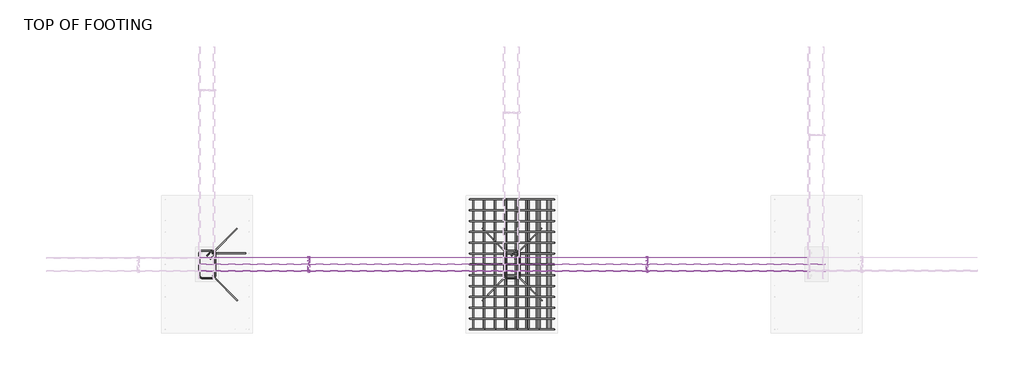
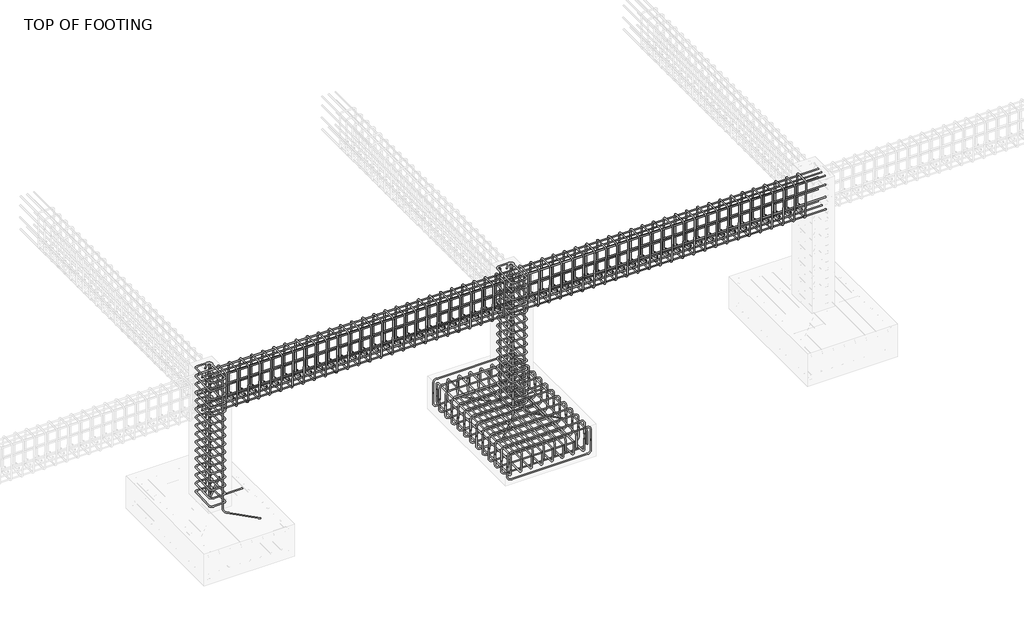
# One storey, part 3 of 21: 28 reinforcing bars.
"""IFC4 building model written with IfcOpenShell, lengths in millimetres."""

from ifc_helpers import new_model, si_unit, point, frame, origin, place, context, project, spatial, polyline, circle_curve, trimmed, segment, composite_curve, source, transform, mapped, element, save
from ifc_brep_helpers import swept_disk

model = new_model("IFC4")

# Units and contexts
model_context = context("Model", 3, world=origin())
ifc_project = project(units=[si_unit("LENGTHUNIT", "METRE", prefix="MILLI")], contexts=[model_context])

# Site, building, storey
site = spatial("IfcSite", under=ifc_project)
building = spatial("IfcBuilding", under=site)
storey = spatial("IfcBuildingStorey", under=building, Name="TOP OF FOOTING", Elevation=-1828.8)

# Reinforcing bars
placement = place(None, origin())
reinforcing_bar_shape = source(origin(), model_context, "Body", "SolidModel", [
    swept_disk(composite_curve([segment(polyline([(-5248.5313539, 443.1886958, -2045.4168622), (-5248.5313539, 443.1886958, -2192.7168622)]), True, "CONTINUOUS"), segment(trimmed(circle_curve(frame((-5294.8813539, 443.1886958, -2192.7168622), z_axis=(0.0, 1.0, 0.0), x_axis=(46.350000000000364, 0.0, 0.0)), 46.35), [point((-5248.5313539, 443.1886958, -2192.7168622))], [point((-5294.8813539, 443.1886958, -2239.0668622))], True, "CARTESIAN"), True, "CONTINUOUS"), segment(polyline([(-5294.8813539, 443.1886958, -2239.0668622), (-6309.4813539, 443.1886958, -2239.0668622)]), True, "CONTINUOUS"), segment(trimmed(circle_curve(frame((-6309.4813539, 443.1886958, -2192.7168622), z_axis=(0.0, 1.0, 0.0), x_axis=(0.0, 0.0, -46.34999999999991)), 46.35), [point((-6309.4813539, 443.1886958, -2239.0668622))], [point((-6355.8313539, 443.1886958, -2192.7168622))], True, "CARTESIAN"), True, "CONTINUOUS"), segment(polyline([(-6355.8313539, 443.1886958, -2192.7168622), (-6355.8313539, 443.1886958, -2045.4168622)]), True, "CONTINUOUS")], self_intersect=False), 6.35),
])
element("IfcReinforcingBar", 1, at=placement, inside=storey, context=model_context, shape_type="MappedRepresentation", body=[
    mapped(reinforcing_bar_shape, transform((0.0, 0.0, 0.0), x_axis=(1.0, 0.0, 0.0), y_axis=(0.0, 1.0, 0.0), z_axis=(0.0, 0.0, 1.0))),
    mapped(reinforcing_bar_shape, transform((0.0, -142.275, 0.0), x_axis=(1.0, 0.0, 0.0), y_axis=(0.0, 1.0, 0.0), z_axis=(0.0, 0.0, 1.0))),
    mapped(reinforcing_bar_shape, transform((0.0, -284.55, 0.0), x_axis=(1.0, 0.0, 0.0), y_axis=(0.0, 1.0, 0.0), z_axis=(0.0, 0.0, 1.0))),
    mapped(reinforcing_bar_shape, transform((0.0, -426.825, 0.0), x_axis=(1.0, 0.0, 0.0), y_axis=(0.0, 1.0, 0.0), z_axis=(0.0, 0.0, 1.0))),
    mapped(reinforcing_bar_shape, transform((0.0, -569.1, 0.0), x_axis=(1.0, 0.0, 0.0), y_axis=(0.0, 1.0, 0.0), z_axis=(0.0, 0.0, 1.0))),
    mapped(reinforcing_bar_shape, transform((0.0, -711.375, 0.0), x_axis=(1.0, 0.0, 0.0), y_axis=(0.0, 1.0, 0.0), z_axis=(0.0, 0.0, 1.0))),
    mapped(reinforcing_bar_shape, transform((0.0, -853.65, 0.0), x_axis=(1.0, 0.0, 0.0), y_axis=(0.0, 1.0, 0.0), z_axis=(0.0, 0.0, 1.0))),
    mapped(reinforcing_bar_shape, transform((0.0, -995.925, 0.0), x_axis=(1.0, 0.0, 0.0), y_axis=(0.0, 1.0, 0.0), z_axis=(0.0, 0.0, 1.0))),
    mapped(reinforcing_bar_shape, transform((0.0, -1138.2, 0.0), x_axis=(1.0, 0.0, 0.0), y_axis=(0.0, 1.0, 0.0), z_axis=(0.0, 0.0, 1.0))),
    mapped(reinforcing_bar_shape, transform((0.0, -1280.475, 0.0), x_axis=(1.0, 0.0, 0.0), y_axis=(0.0, 1.0, 0.0), z_axis=(0.0, 0.0, 1.0))),
    mapped(reinforcing_bar_shape, transform((0.0, -1422.75, 0.0), x_axis=(1.0, 0.0, 0.0), y_axis=(0.0, 1.0, 0.0), z_axis=(0.0, 0.0, 1.0))),
    mapped(reinforcing_bar_shape, transform((0.0, -1565.025, 0.0), x_axis=(1.0, 0.0, 0.0), y_axis=(0.0, 1.0, 0.0), z_axis=(0.0, 0.0, 1.0))),
    mapped(reinforcing_bar_shape, transform((0.0, -1707.3, 0.0), x_axis=(1.0, 0.0, 0.0), y_axis=(0.0, 1.0, 0.0), z_axis=(0.0, 0.0, 1.0))),
])
reinforcing_bar_2_shape = source(origin(), model_context, "Body", "SolidModel", [
    swept_disk(composite_curve([segment(polyline([(-6352.5002917, 443.1886958, -2057.1074344), (-6352.5002917, 443.1886958, -1909.8074344)]), True, "CONTINUOUS"), segment(trimmed(circle_curve(frame((-6306.1502917, 443.1886958, -1909.8074344), z_axis=(0.0, 1.0, 0.0), x_axis=(-46.350000000000364, 0.0, 0.0)), 46.35), [point((-6352.5002917, 443.1886958, -1909.8074344))], [point((-6306.1502917, 443.1886958, -1863.4574344))], True, "CARTESIAN"), True, "CONTINUOUS"), segment(polyline([(-6306.1502917, 443.1886958, -1863.4574344), (-5297.2599214, 443.1886958, -1863.4574344)]), True, "CONTINUOUS"), segment(trimmed(circle_curve(frame((-5297.2599214, 443.1886958, -1909.8074344), z_axis=(0.0, 1.0, 0.0), x_axis=(0.0, 0.0, 46.34999999999991)), 46.35), [point((-5297.2599214, 443.1886958, -1863.4574344))], [point((-5250.9099214, 443.1886958, -1909.8074344))], True, "CARTESIAN"), True, "CONTINUOUS"), segment(polyline([(-5250.9099214, 443.1886958, -1909.8074344), (-5250.9099214, 443.1886958, -2057.1074344)]), True, "CONTINUOUS")], self_intersect=False), 6.35),
])
element("IfcReinforcingBar", 2, at=placement, inside=storey, context=model_context, shape_type="MappedRepresentation", body=[
    mapped(reinforcing_bar_2_shape, transform((0.0, 0.0, 0.0), x_axis=(1.0, 0.0, 0.0), y_axis=(0.0, 1.0, 0.0), z_axis=(0.0, 0.0, 1.0))),
    mapped(reinforcing_bar_2_shape, transform((0.0, -142.275, 0.0), x_axis=(1.0, 0.0, 0.0), y_axis=(0.0, 1.0, 0.0), z_axis=(0.0, 0.0, 1.0))),
    mapped(reinforcing_bar_2_shape, transform((0.0, -284.55, 0.0), x_axis=(1.0, 0.0, 0.0), y_axis=(0.0, 1.0, 0.0), z_axis=(0.0, 0.0, 1.0))),
    mapped(reinforcing_bar_2_shape, transform((0.0, -426.825, 0.0), x_axis=(1.0, 0.0, 0.0), y_axis=(0.0, 1.0, 0.0), z_axis=(0.0, 0.0, 1.0))),
    mapped(reinforcing_bar_2_shape, transform((0.0, -569.1, 0.0), x_axis=(1.0, 0.0, 0.0), y_axis=(0.0, 1.0, 0.0), z_axis=(0.0, 0.0, 1.0))),
    mapped(reinforcing_bar_2_shape, transform((0.0, -711.375, 0.0), x_axis=(1.0, 0.0, 0.0), y_axis=(0.0, 1.0, 0.0), z_axis=(0.0, 0.0, 1.0))),
    mapped(reinforcing_bar_2_shape, transform((0.0, -853.65, 0.0), x_axis=(1.0, 0.0, 0.0), y_axis=(0.0, 1.0, 0.0), z_axis=(0.0, 0.0, 1.0))),
    mapped(reinforcing_bar_2_shape, transform((0.0, -995.925, 0.0), x_axis=(1.0, 0.0, 0.0), y_axis=(0.0, 1.0, 0.0), z_axis=(0.0, 0.0, 1.0))),
    mapped(reinforcing_bar_2_shape, transform((0.0, -1138.2, 0.0), x_axis=(1.0, 0.0, 0.0), y_axis=(0.0, 1.0, 0.0), z_axis=(0.0, 0.0, 1.0))),
    mapped(reinforcing_bar_2_shape, transform((0.0, -1280.475, 0.0), x_axis=(1.0, 0.0, 0.0), y_axis=(0.0, 1.0, 0.0), z_axis=(0.0, 0.0, 1.0))),
    mapped(reinforcing_bar_2_shape, transform((0.0, -1422.75, 0.0), x_axis=(1.0, 0.0, 0.0), y_axis=(0.0, 1.0, 0.0), z_axis=(0.0, 0.0, 1.0))),
    mapped(reinforcing_bar_2_shape, transform((0.0, -1565.025, 0.0), x_axis=(1.0, 0.0, 0.0), y_axis=(0.0, 1.0, 0.0), z_axis=(0.0, 0.0, 1.0))),
    mapped(reinforcing_bar_2_shape, transform((0.0, -1707.3, 0.0), x_axis=(1.0, 0.0, 0.0), y_axis=(0.0, 1.0, 0.0), z_axis=(0.0, 0.0, 1.0))),
])
reinforcing_bar_3_shape = source(origin(), model_context, "Body", "SolidModel", [
    swept_disk(composite_curve([segment(polyline([(-5294.4849216, 443.1886958, -2099.3509187), (-5294.4849216, 443.1886958, -1952.0509187)]), True, "CONTINUOUS"), segment(trimmed(circle_curve(frame((-5294.4849216, 396.8386958, -1952.0509187), z_axis=(1.0, 0.0, 0.0), x_axis=(0.0, 46.35000000000002, 0.0)), 46.35), [point((-5294.4849216, 443.1886958, -1952.0509187))], [point((-5294.4849216, 396.8386958, -1905.7009187))], True, "CARTESIAN"), True, "CONTINUOUS"), segment(polyline([(-5294.4849216, 396.8386958, -1905.7009187), (-5294.4849216, -1217.7613042, -1905.7009187)]), True, "CONTINUOUS"), segment(trimmed(circle_curve(frame((-5294.4849216, -1217.7613042, -1952.0509187), z_axis=(1.0, 0.0, 0.0), x_axis=(0.0, 0.0, 46.34999999999991)), 46.35), [point((-5294.4849216, -1217.7613042, -1905.7009187))], [point((-5294.4849216, -1264.1113042, -1952.0509187))], True, "CARTESIAN"), True, "CONTINUOUS"), segment(polyline([(-5294.4849216, -1264.1113042, -1952.0509187), (-5294.4849216, -1264.1113042, -2099.3509187)]), True, "CONTINUOUS")], self_intersect=False), 6.35),
])
element("IfcReinforcingBar", 3, at=placement, inside=storey, context=model_context, shape_type="MappedRepresentation", body=[
    mapped(reinforcing_bar_3_shape, transform((0.0, 0.0, 0.0), x_axis=(1.0, 0.0, 0.0), y_axis=(0.0, 1.0, 0.0), z_axis=(0.0, 0.0, 1.0))),
    mapped(reinforcing_bar_3_shape, transform((-145.0295561, 0.0, 0.0), x_axis=(1.0, 0.0, 0.0), y_axis=(0.0, 1.0, 0.0), z_axis=(0.0, 0.0, 1.0))),
    mapped(reinforcing_bar_3_shape, transform((-290.0591123, 0.0, 0.0), x_axis=(1.0, 0.0, 0.0), y_axis=(0.0, 1.0, 0.0), z_axis=(0.0, 0.0, 1.0))),
    mapped(reinforcing_bar_3_shape, transform((-435.0886684, 0.0, 0.0), x_axis=(1.0, 0.0, 0.0), y_axis=(0.0, 1.0, 0.0), z_axis=(0.0, 0.0, 1.0))),
    mapped(reinforcing_bar_3_shape, transform((-580.1182245, 0.0, 0.0), x_axis=(1.0, 0.0, 0.0), y_axis=(0.0, 1.0, 0.0), z_axis=(0.0, 0.0, 1.0))),
    mapped(reinforcing_bar_3_shape, transform((-725.1477807, 0.0, 0.0), x_axis=(1.0, 0.0, 0.0), y_axis=(0.0, 1.0, 0.0), z_axis=(0.0, 0.0, 1.0))),
    mapped(reinforcing_bar_3_shape, transform((-870.1773368, 0.0, 0.0), x_axis=(1.0, 0.0, 0.0), y_axis=(0.0, 1.0, 0.0), z_axis=(0.0, 0.0, 1.0))),
    mapped(reinforcing_bar_3_shape, transform((-1015.206893, 0.0, 0.0), x_axis=(1.0, 0.0, 0.0), y_axis=(0.0, 1.0, 0.0), z_axis=(0.0, 0.0, 1.0))),
])
reinforcing_bar_4_shape = source(origin(), model_context, "Body", "SolidModel", [
    swept_disk(composite_curve([segment(polyline([(-6309.6918146, 443.1886958, -2006.0306816), (-6309.6918146, 443.1886958, -2153.3306816)]), True, "CONTINUOUS"), segment(trimmed(circle_curve(frame((-6309.6918146, 396.8386958, -2153.3306816), z_axis=(-1.0, 0.0, 0.0), x_axis=(0.0, 46.35000000000002, 0.0)), 46.35), [point((-6309.6918146, 443.1886958, -2153.3306816))], [point((-6309.6918146, 396.8386958, -2199.6806816))], True, "CARTESIAN"), True, "CONTINUOUS"), segment(polyline([(-6309.6918146, 396.8386958, -2199.6806816), (-6309.6918146, -1217.7613042, -2199.6806816)]), True, "CONTINUOUS"), segment(trimmed(circle_curve(frame((-6309.6918146, -1217.7613042, -2153.3306816), z_axis=(-1.0, 0.0, 0.0), x_axis=(0.0, 0.0, -46.34999999999991)), 46.35), [point((-6309.6918146, -1217.7613042, -2199.6806816))], [point((-6309.6918146, -1264.1113042, -2153.3306816))], True, "CARTESIAN"), True, "CONTINUOUS"), segment(polyline([(-6309.6918146, -1264.1113042, -2153.3306816), (-6309.6918146, -1264.1113042, -2006.0306816)]), True, "CONTINUOUS")], self_intersect=False), 6.35),
])
element("IfcReinforcingBar", 4, at=placement, inside=storey, context=model_context, shape_type="MappedRepresentation", body=[
    mapped(reinforcing_bar_4_shape, transform((0.0, 0.0, 0.0), x_axis=(1.0, 0.0, 0.0), y_axis=(0.0, 1.0, 0.0), z_axis=(0.0, 0.0, 1.0))),
    mapped(reinforcing_bar_4_shape, transform((138.8823255, 0.0, 0.0), x_axis=(1.0, 0.0, 0.0), y_axis=(0.0, 1.0, 0.0), z_axis=(0.0, 0.0, 1.0))),
    mapped(reinforcing_bar_4_shape, transform((277.7646509, 0.0, 0.0), x_axis=(1.0, 0.0, 0.0), y_axis=(0.0, 1.0, 0.0), z_axis=(0.0, 0.0, 1.0))),
    mapped(reinforcing_bar_4_shape, transform((416.6469764, 0.0, 0.0), x_axis=(1.0, 0.0, 0.0), y_axis=(0.0, 1.0, 0.0), z_axis=(0.0, 0.0, 1.0))),
    mapped(reinforcing_bar_4_shape, transform((555.5293018, 0.0, 0.0), x_axis=(1.0, 0.0, 0.0), y_axis=(0.0, 1.0, 0.0), z_axis=(0.0, 0.0, 1.0))),
    mapped(reinforcing_bar_4_shape, transform((694.4116273, 0.0, 0.0), x_axis=(1.0, 0.0, 0.0), y_axis=(0.0, 1.0, 0.0), z_axis=(0.0, 0.0, 1.0))),
    mapped(reinforcing_bar_4_shape, transform((833.2939527, 0.0, 0.0), x_axis=(1.0, 0.0, 0.0), y_axis=(0.0, 1.0, 0.0), z_axis=(0.0, 0.0, 1.0))),
    mapped(reinforcing_bar_4_shape, transform((972.1762782, 0.0, 0.0), x_axis=(1.0, 0.0, 0.0), y_axis=(0.0, 1.0, 0.0), z_axis=(0.0, 0.0, 1.0))),
])
reinforcing_bar_5_shape = source(origin(), model_context, "Body", "SolidModel", [
    swept_disk(composite_curve([segment(polyline([(-9807.7927145, -296.7370695, -46.35), (-9752.0491515, -240.9935066, -46.35)]), True, "CONTINUOUS"), segment(trimmed(circle_curve(frame((-9729.8813539, -263.1613042, -46.35), z_axis=(0.0, 0.0, -1.0), x_axis=(-22.167797599999176, 22.16779760000003, 0.0)), 31.35), [point((-9752.0491515, -240.9935066, -46.35))], [point((-9698.5313539, -263.1613042, -46.35))], True, "CARTESIAN"), True, "CONTINUOUS"), segment(polyline([(-9698.5313539, -263.1613042, -46.35), (-9698.5313539, -557.7613042, -46.35)]), True, "CONTINUOUS"), segment(trimmed(circle_curve(frame((-9729.8813539, -557.7613042, -46.35), z_axis=(0.0, 0.0, -1.0), x_axis=(31.350000000000364, 0.0, 0.0)), 31.35), [point((-9698.5313539, -557.7613042, -46.35))], [point((-9729.8813539, -589.1113042, -46.35))], True, "CARTESIAN"), True, "CONTINUOUS"), segment(polyline([(-9729.8813539, -589.1113042, -46.35), (-9874.4813539, -589.1113042, -46.35)]), True, "CONTINUOUS"), segment(trimmed(circle_curve(frame((-9874.4813539, -557.7810893, -45.2363875), z_axis=(0.0, 0.035521928334481916, -0.9993688971583016), x_axis=(0.0, -31.330214899999987, -1.1136125000000021)), 31.35), [point((-9874.4813539, -589.1113042, -46.35))], [point((-9905.8313539, -557.7810893, -45.2363875))], True, "CARTESIAN"), True, "CONTINUOUS"), segment(polyline([(-9905.8313539, -557.7810893, -45.2363875), (-9905.8313539, -263.1415191, -34.7636125)]), True, "CONTINUOUS"), segment(trimmed(circle_curve(frame((-9874.4813539, -263.1415191, -34.7636125), z_axis=(0.0, 0.035521928334481916, -0.9993688971583016), x_axis=(-31.349999999998545, 0.0, 0.0)), 31.35), [point((-9905.8313539, -263.1415191, -34.7636125))], [point((-9874.4813539, -231.8113042, -33.65))], True, "CARTESIAN"), True, "CONTINUOUS"), segment(polyline([(-9874.4813539, -231.8113042, -33.65), (-9729.8813539, -231.8113042, -33.65)]), True, "CONTINUOUS"), segment(trimmed(circle_curve(frame((-9729.8813539, -263.1613042, -33.65), z_axis=(0.0, 0.0, -1.0), x_axis=(0.0, 31.350000000000023, 0.0)), 31.35), [point((-9729.8813539, -231.8113042, -33.65))], [point((-9707.7135563, -285.3291018, -33.65))], True, "CARTESIAN"), True, "CONTINUOUS"), segment(polyline([(-9707.7135563, -285.3291018, -33.65), (-9763.4571193, -341.0726647, -33.65)]), True, "CONTINUOUS")], self_intersect=False), 6.35),
])
element("IfcReinforcingBar", 5, at=placement, inside=storey, context=model_context, shape_type="MappedRepresentation", body=[
    mapped(reinforcing_bar_5_shape, transform((0.0, 0.0, 0.0), x_axis=(1.0, 0.0, 0.0), y_axis=(0.0, 1.0, 0.0), z_axis=(0.0, 0.0, 1.0))),
    mapped(reinforcing_bar_5_shape, transform((0.0, 0.0, -115.74), x_axis=(1.0, 0.0, 0.0), y_axis=(0.0, 1.0, 0.0), z_axis=(0.0, 0.0, 1.0))),
    mapped(reinforcing_bar_5_shape, transform((0.0, 0.0, -231.48), x_axis=(1.0, 0.0, 0.0), y_axis=(0.0, 1.0, 0.0), z_axis=(0.0, 0.0, 1.0))),
    mapped(reinforcing_bar_5_shape, transform((0.0, 0.0, -347.22), x_axis=(1.0, 0.0, 0.0), y_axis=(0.0, 1.0, 0.0), z_axis=(0.0, 0.0, 1.0))),
    mapped(reinforcing_bar_5_shape, transform((0.0, 0.0, -462.96), x_axis=(1.0, 0.0, 0.0), y_axis=(0.0, 1.0, 0.0), z_axis=(0.0, 0.0, 1.0))),
    mapped(reinforcing_bar_5_shape, transform((0.0, 0.0, -578.7), x_axis=(1.0, 0.0, 0.0), y_axis=(0.0, 1.0, 0.0), z_axis=(0.0, 0.0, 1.0))),
    mapped(reinforcing_bar_5_shape, transform((0.0, 0.0, -694.44), x_axis=(1.0, 0.0, 0.0), y_axis=(0.0, 1.0, 0.0), z_axis=(0.0, 0.0, 1.0))),
    mapped(reinforcing_bar_5_shape, transform((0.0, 0.0, -810.18), x_axis=(1.0, 0.0, 0.0), y_axis=(0.0, 1.0, 0.0), z_axis=(0.0, 0.0, 1.0))),
    mapped(reinforcing_bar_5_shape, transform((0.0, 0.0, -925.92), x_axis=(1.0, 0.0, 0.0), y_axis=(0.0, 1.0, 0.0), z_axis=(0.0, 0.0, 1.0))),
    mapped(reinforcing_bar_5_shape, transform((0.0, 0.0, -1041.66), x_axis=(1.0, 0.0, 0.0), y_axis=(0.0, 1.0, 0.0), z_axis=(0.0, 0.0, 1.0))),
    mapped(reinforcing_bar_5_shape, transform((0.0, 0.0, -1157.4), x_axis=(1.0, 0.0, 0.0), y_axis=(0.0, 1.0, 0.0), z_axis=(0.0, 0.0, 1.0))),
    mapped(reinforcing_bar_5_shape, transform((0.0, 0.0, -1273.14), x_axis=(1.0, 0.0, 0.0), y_axis=(0.0, 1.0, 0.0), z_axis=(0.0, 0.0, 1.0))),
    mapped(reinforcing_bar_5_shape, transform((0.0, 0.0, -1388.88), x_axis=(1.0, 0.0, 0.0), y_axis=(0.0, 1.0, 0.0), z_axis=(0.0, 0.0, 1.0))),
    mapped(reinforcing_bar_5_shape, transform((0.0, 0.0, -1504.62), x_axis=(1.0, 0.0, 0.0), y_axis=(0.0, 1.0, 0.0), z_axis=(0.0, 0.0, 1.0))),
    mapped(reinforcing_bar_5_shape, transform((0.0, 0.0, -1620.36), x_axis=(1.0, 0.0, 0.0), y_axis=(0.0, 1.0, 0.0), z_axis=(0.0, 0.0, 1.0))),
    mapped(reinforcing_bar_5_shape, transform((0.0, 0.0, -1736.1), x_axis=(1.0, 0.0, 0.0), y_axis=(0.0, 1.0, 0.0), z_axis=(0.0, 0.0, 1.0))),
])
element("IfcReinforcingBar", 6, at=placement, inside=storey, context=model_context, shape_type="SolidModel", body=[
    swept_disk(composite_curve([segment(polyline([(-9730.3607537, -262.059512, -40.0), (-9730.3607537, -262.059512, -1882.5259187)]), True, "CONTINUOUS"), segment(trimmed(circle_curve(frame((-9684.0107537, -262.059512, -1882.5259187), z_axis=(0.0, -1.0, 0.0), x_axis=(-46.350000000000364, 0.0, 0.0)), 46.35), [point((-9730.3607537, -262.059512, -1882.5259187))], [point((-9684.0107537, -262.059512, -1928.8759187))], True, "CARTESIAN"), True, "CONTINUOUS"), segment(polyline([(-9684.0107537, -262.059512, -1928.8759187), (-9294.4849216, -262.059512, -1928.8759187)]), True, "CONTINUOUS")], self_intersect=False), 6.35),
])
element("IfcReinforcingBar", 7, at=placement, inside=storey, context=model_context, shape_type="SolidModel", body=[
    swept_disk(composite_curve([segment(polyline([(-9730.3607537, -262.059512, -40.0), (-9730.3607537, -262.059512, -1882.5259187)]), True, "CONTINUOUS"), segment(trimmed(circle_curve(frame((-9697.9026361, -228.9718542, -1882.5259187), z_axis=(0.7138653253877265, -0.7002830122236834, 0.0), x_axis=(-32.45811760000106, -33.08765779999999, 0.0)), 46.35), [point((-9730.3607537, -262.059512, -1882.5259187))], [point((-9697.9026361, -228.9718542, -1928.8759187))], True, "CARTESIAN"), True, "CONTINUOUS"), segment(polyline([(-9697.9026361, -228.9718542, -1928.8759187), (-9413.1331156, 61.320903, -1928.8759187)]), True, "CONTINUOUS")], self_intersect=False), 6.35),
])
element("IfcReinforcingBar", 8, at=placement, inside=storey, context=model_context, shape_type="SolidModel", body=[
    swept_disk(composite_curve([segment(polyline([(-9725.3607537, -561.3630964, -40.0), (-9725.3607537, -561.3630964, -1882.5259187)]), True, "CONTINUOUS"), segment(trimmed(circle_curve(frame((-9692.9026361, -594.4507542, -1882.5259187), z_axis=(-0.7138653253877265, -0.7002830122236834, 0.0), x_axis=(-32.45811760000106, 33.08765779999999, 0.0)), 46.35), [point((-9725.3607537, -561.3630964, -1882.5259187))], [point((-9692.9026361, -594.4507542, -1928.8759187))], True, "CARTESIAN"), True, "CONTINUOUS"), segment(polyline([(-9692.9026361, -594.4507542, -1928.8759187), (-9408.1331156, -884.7435113, -1928.8759187)]), True, "CONTINUOUS")], self_intersect=False), 6.35),
])
reinforcing_bar_6_shape = source(origin(), model_context, "Body", "SolidModel", [
    swept_disk(composite_curve([segment(polyline([(-5807.7927145, -296.7370695, -46.35), (-5752.0491515, -240.9935066, -46.35)]), True, "CONTINUOUS"), segment(trimmed(circle_curve(frame((-5729.8813539, -263.1613042, -46.35), z_axis=(0.0, 0.0, -1.0), x_axis=(-22.167797600000085, 22.16779760000003, 0.0)), 31.35), [point((-5752.0491515, -240.9935066, -46.35))], [point((-5698.5313539, -263.1613042, -46.35))], True, "CARTESIAN"), True, "CONTINUOUS"), segment(polyline([(-5698.5313539, -263.1613042, -46.35), (-5698.5313539, -557.7613042, -46.35)]), True, "CONTINUOUS"), segment(trimmed(circle_curve(frame((-5729.8813539, -557.7613042, -46.35), z_axis=(0.0, 0.0, -1.0), x_axis=(31.350000000000364, 0.0, 0.0)), 31.35), [point((-5698.5313539, -557.7613042, -46.35))], [point((-5729.8813539, -589.1113042, -46.35))], True, "CARTESIAN"), True, "CONTINUOUS"), segment(polyline([(-5729.8813539, -589.1113042, -46.35), (-5874.4813539, -589.1113042, -46.35)]), True, "CONTINUOUS"), segment(trimmed(circle_curve(frame((-5874.4813539, -557.7810893, -45.2363875), z_axis=(0.0, 0.035521928334481916, -0.9993688971583016), x_axis=(0.0, -31.330214899999987, -1.1136125000000021)), 31.35), [point((-5874.4813539, -589.1113042, -46.35))], [point((-5905.8313539, -557.7810893, -45.2363875))], True, "CARTESIAN"), True, "CONTINUOUS"), segment(polyline([(-5905.8313539, -557.7810893, -45.2363875), (-5905.8313539, -263.1415191, -34.7636125)]), True, "CONTINUOUS"), segment(trimmed(circle_curve(frame((-5874.4813539, -263.1415191, -34.7636125), z_axis=(0.0, 0.035521928334481916, -0.9993688971583016), x_axis=(-31.350000000000364, 0.0, 0.0)), 31.35), [point((-5905.8313539, -263.1415191, -34.7636125))], [point((-5874.4813539, -231.8113042, -33.65))], True, "CARTESIAN"), True, "CONTINUOUS"), segment(polyline([(-5874.4813539, -231.8113042, -33.65), (-5729.8813539, -231.8113042, -33.65)]), True, "CONTINUOUS"), segment(trimmed(circle_curve(frame((-5729.8813539, -263.1613042, -33.65), z_axis=(0.0, 0.0, -1.0), x_axis=(0.0, 31.350000000000023, 0.0)), 31.35), [point((-5729.8813539, -231.8113042, -33.65))], [point((-5707.7135563, -285.3291018, -33.65))], True, "CARTESIAN"), True, "CONTINUOUS"), segment(polyline([(-5707.7135563, -285.3291018, -33.65), (-5763.4571193, -341.0726647, -33.65)]), True, "CONTINUOUS")], self_intersect=False), 6.35),
])
element("IfcReinforcingBar", 9, at=placement, inside=storey, context=model_context, shape_type="MappedRepresentation", body=[
    mapped(reinforcing_bar_6_shape, transform((0.0, 0.0, 0.0), x_axis=(1.0, 0.0, 0.0), y_axis=(0.0, 1.0, 0.0), z_axis=(0.0, 0.0, 1.0))),
    mapped(reinforcing_bar_6_shape, transform((0.0, 0.0, -115.74), x_axis=(1.0, 0.0, 0.0), y_axis=(0.0, 1.0, 0.0), z_axis=(0.0, 0.0, 1.0))),
    mapped(reinforcing_bar_6_shape, transform((0.0, 0.0, -231.48), x_axis=(1.0, 0.0, 0.0), y_axis=(0.0, 1.0, 0.0), z_axis=(0.0, 0.0, 1.0))),
    mapped(reinforcing_bar_6_shape, transform((0.0, 0.0, -347.22), x_axis=(1.0, 0.0, 0.0), y_axis=(0.0, 1.0, 0.0), z_axis=(0.0, 0.0, 1.0))),
    mapped(reinforcing_bar_6_shape, transform((0.0, 0.0, -462.96), x_axis=(1.0, 0.0, 0.0), y_axis=(0.0, 1.0, 0.0), z_axis=(0.0, 0.0, 1.0))),
    mapped(reinforcing_bar_6_shape, transform((0.0, 0.0, -578.7), x_axis=(1.0, 0.0, 0.0), y_axis=(0.0, 1.0, 0.0), z_axis=(0.0, 0.0, 1.0))),
    mapped(reinforcing_bar_6_shape, transform((0.0, 0.0, -694.44), x_axis=(1.0, 0.0, 0.0), y_axis=(0.0, 1.0, 0.0), z_axis=(0.0, 0.0, 1.0))),
    mapped(reinforcing_bar_6_shape, transform((0.0, 0.0, -810.18), x_axis=(1.0, 0.0, 0.0), y_axis=(0.0, 1.0, 0.0), z_axis=(0.0, 0.0, 1.0))),
    mapped(reinforcing_bar_6_shape, transform((0.0, 0.0, -925.92), x_axis=(1.0, 0.0, 0.0), y_axis=(0.0, 1.0, 0.0), z_axis=(0.0, 0.0, 1.0))),
    mapped(reinforcing_bar_6_shape, transform((0.0, 0.0, -1041.66), x_axis=(1.0, 0.0, 0.0), y_axis=(0.0, 1.0, 0.0), z_axis=(0.0, 0.0, 1.0))),
    mapped(reinforcing_bar_6_shape, transform((0.0, 0.0, -1157.4), x_axis=(1.0, 0.0, 0.0), y_axis=(0.0, 1.0, 0.0), z_axis=(0.0, 0.0, 1.0))),
    mapped(reinforcing_bar_6_shape, transform((0.0, 0.0, -1273.14), x_axis=(1.0, 0.0, 0.0), y_axis=(0.0, 1.0, 0.0), z_axis=(0.0, 0.0, 1.0))),
    mapped(reinforcing_bar_6_shape, transform((0.0, 0.0, -1388.88), x_axis=(1.0, 0.0, 0.0), y_axis=(0.0, 1.0, 0.0), z_axis=(0.0, 0.0, 1.0))),
    mapped(reinforcing_bar_6_shape, transform((0.0, 0.0, -1504.62), x_axis=(1.0, 0.0, 0.0), y_axis=(0.0, 1.0, 0.0), z_axis=(0.0, 0.0, 1.0))),
    mapped(reinforcing_bar_6_shape, transform((0.0, 0.0, -1620.36), x_axis=(1.0, 0.0, 0.0), y_axis=(0.0, 1.0, 0.0), z_axis=(0.0, 0.0, 1.0))),
    mapped(reinforcing_bar_6_shape, transform((0.0, 0.0, -1736.1), x_axis=(1.0, 0.0, 0.0), y_axis=(0.0, 1.0, 0.0), z_axis=(0.0, 0.0, 1.0))),
])
element("IfcReinforcingBar", 10, at=placement, inside=storey, context=model_context, shape_type="SolidModel", body=[
    swept_disk(composite_curve([segment(polyline([(-5730.3607537, -262.059512, -40.0), (-5730.3607537, -262.059512, -1882.5259187)]), True, "CONTINUOUS"), segment(trimmed(circle_curve(frame((-5684.0107537, -262.059512, -1882.5259187), z_axis=(0.0, -1.0, 0.0), x_axis=(-46.349999999999454, 0.0, 0.0)), 46.35), [point((-5730.3607537, -262.059512, -1882.5259187))], [point((-5684.0107537, -262.059512, -1928.8759187))], True, "CARTESIAN"), True, "CONTINUOUS"), segment(polyline([(-5684.0107537, -262.059512, -1928.8759187), (-5294.4849216, -262.059512, -1928.8759187)]), True, "CONTINUOUS")], self_intersect=False), 6.35),
])
element("IfcReinforcingBar", 11, at=placement, inside=storey, context=model_context, shape_type="SolidModel", body=[
    swept_disk(composite_curve([segment(polyline([(-5730.3607537, -262.059512, -40.0), (-5730.3607537, -262.059512, -1882.5259187)]), True, "CONTINUOUS"), segment(trimmed(circle_curve(frame((-5697.9026361, -228.9718542, -1882.5259187), z_axis=(0.7138653253877265, -0.7002830122236834, 0.0), x_axis=(-32.45811760000015, -33.08765779999999, 0.0)), 46.35), [point((-5730.3607537, -262.059512, -1882.5259187))], [point((-5697.9026361, -228.9718542, -1928.8759187))], True, "CARTESIAN"), True, "CONTINUOUS"), segment(polyline([(-5697.9026361, -228.9718542, -1928.8759187), (-5413.1331156, 61.320903, -1928.8759187)]), True, "CONTINUOUS")], self_intersect=False), 6.35),
])
element("IfcReinforcingBar", 12, at=placement, inside=storey, context=model_context, shape_type="SolidModel", body=[
    swept_disk(composite_curve([segment(polyline([(-5874.0019542, -262.059512, -40.0), (-5874.0019542, -262.059512, -1882.5259187)]), True, "CONTINUOUS"), segment(trimmed(circle_curve(frame((-5906.4600718, -228.9718542, -1882.5259187), z_axis=(0.7138653253877092, 0.700283012223701, 0.0), x_axis=(32.45811760000015, -33.08765779999999, 0.0)), 46.35), [point((-5874.0019542, -262.059512, -1882.5259187))], [point((-5906.4600718, -228.9718542, -1928.8759187))], True, "CARTESIAN"), True, "CONTINUOUS"), segment(polyline([(-5906.4600718, -228.9718542, -1928.8759187), (-6191.2295922, 61.320903, -1928.8759187)]), True, "CONTINUOUS")], self_intersect=False), 6.35),
])
element("IfcReinforcingBar", 13, at=placement, inside=storey, context=model_context, shape_type="SolidModel", body=[
    swept_disk(composite_curve([segment(polyline([(-5725.3607537, -561.3630964, -40.0), (-5725.3607537, -561.3630964, -1882.5259187)]), True, "CONTINUOUS"), segment(trimmed(circle_curve(frame((-5692.9026361, -594.4507542, -1882.5259187), z_axis=(-0.7138653253877265, -0.7002830122236834, 0.0), x_axis=(-32.45811760000015, 33.08765779999999, 0.0)), 46.35), [point((-5725.3607537, -561.3630964, -1882.5259187))], [point((-5692.9026361, -594.4507542, -1928.8759187))], True, "CARTESIAN"), True, "CONTINUOUS"), segment(polyline([(-5692.9026361, -594.4507542, -1928.8759187), (-5408.1331156, -884.7435113, -1928.8759187)]), True, "CONTINUOUS")], self_intersect=False), 6.35),
])
element("IfcReinforcingBar", 14, at=placement, inside=storey, context=model_context, shape_type="SolidModel", body=[
    swept_disk(composite_curve([segment(polyline([(-5874.0019542, -558.8630964, -40.0), (-5874.0019542, -558.8630964, -1882.5259187)]), True, "CONTINUOUS"), segment(trimmed(circle_curve(frame((-5906.4600718, -591.9507542, -1882.5259187), z_axis=(-0.7138653253877092, 0.700283012223701, 0.0), x_axis=(32.45811760000015, 33.08765779999999, 0.0)), 46.35), [point((-5874.0019542, -558.8630964, -1882.5259187))], [point((-5906.4600718, -591.9507542, -1928.8759187))], True, "CARTESIAN"), True, "CONTINUOUS"), segment(polyline([(-5906.4600718, -591.9507542, -1928.8759187), (-6191.2295922, -882.2435113, -1928.8759187)]), True, "CONTINUOUS")], self_intersect=False), 6.35),
])
reinforcing_bar_7_shape = source(origin(), model_context, "Body", "SolidModel", [
    swept_disk(composite_curve([segment(polyline([(-5645.8313539, -416.0726647, -488.7242346), (-5645.8313539, -360.3291018, -544.4677976)]), True, "CONTINUOUS"), segment(trimmed(circle_curve(frame((-5645.8313539, -338.1613042, -522.3), z_axis=(1.0, 0.0, 0.0), x_axis=(0.0, -22.16779759999997, -22.167797600000085)), 31.35), [point((-5645.8313539, -360.3291018, -544.4677976))], [point((-5645.8313539, -306.8113042, -522.3))], True, "CARTESIAN"), True, "CONTINUOUS"), segment(polyline([(-5645.8313539, -306.8113042, -522.3), (-5645.8313539, -306.8113042, -77.7)]), True, "CONTINUOUS"), segment(trimmed(circle_curve(frame((-5645.8313539, -338.1613042, -77.7), z_axis=(1.0, 0.0, 0.0), x_axis=(0.0, 31.350000000000023, 0.0)), 31.35), [point((-5645.8313539, -306.8113042, -77.7))], [point((-5645.8313539, -338.1613042, -46.35))], True, "CARTESIAN"), True, "CONTINUOUS"), segment(polyline([(-5645.8313539, -338.1613042, -46.35), (-5645.8313539, -482.7613042, -46.35)]), True, "CONTINUOUS"), segment(trimmed(circle_curve(frame((-5646.6159396, -482.7613042, -77.6901807), z_axis=(0.9996867842138424, 0.0, -0.025026655153786322), x_axis=(0.784585700000207, 0.0, 31.340180699999998)), 31.35), [point((-5645.8313539, -482.7613042, -46.35))], [point((-5646.6159396, -514.1113042, -77.6901807))], True, "CARTESIAN"), True, "CONTINUOUS"), segment(polyline([(-5646.6159396, -514.1113042, -77.6901807), (-5657.7467683, -514.1113042, -522.3098193)]), True, "CONTINUOUS"), segment(trimmed(circle_curve(frame((-5657.7467683, -482.7613042, -522.3098193), z_axis=(0.9996867842138424, 0.0, -0.025026655153786322), x_axis=(0.0, -31.349999999999966, 0.0)), 31.35), [point((-5657.7467683, -514.1113042, -522.3098193))], [point((-5658.5313539, -482.7613042, -553.65))], True, "CARTESIAN"), True, "CONTINUOUS"), segment(polyline([(-5658.5313539, -482.7613042, -553.65), (-5658.5313539, -338.1613042, -553.65)]), True, "CONTINUOUS"), segment(trimmed(circle_curve(frame((-5658.5313539, -338.1613042, -522.3), z_axis=(1.0, 0.0, 0.0), x_axis=(0.0, 0.0, -31.350000000000023)), 31.35), [point((-5658.5313539, -338.1613042, -553.65))], [point((-5658.5313539, -315.9935066, -500.1322024))], True, "CARTESIAN"), True, "CONTINUOUS"), segment(polyline([(-5658.5313539, -315.9935066, -500.1322024), (-5658.5313539, -371.7370695, -444.3886395)]), True, "CONTINUOUS")], self_intersect=False), 6.35),
])
element("IfcReinforcingBar", 15, at=placement, inside=storey, context=model_context, shape_type="MappedRepresentation", body=[
    mapped(reinforcing_bar_7_shape, transform((0.0, 0.0, 0.0), x_axis=(1.0, 0.0, 0.0), y_axis=(0.0, 1.0, 0.0), z_axis=(0.0, 0.0, 1.0))),
    mapped(reinforcing_bar_7_shape, transform((147.492, 0.0, 0.0), x_axis=(1.0, 0.0, 0.0), y_axis=(0.0, 1.0, 0.0), z_axis=(0.0, 0.0, 1.0))),
    mapped(reinforcing_bar_7_shape, transform((294.984, 0.0, 0.0), x_axis=(1.0, 0.0, 0.0), y_axis=(0.0, 1.0, 0.0), z_axis=(0.0, 0.0, 1.0))),
    mapped(reinforcing_bar_7_shape, transform((442.476, 0.0, 0.0), x_axis=(1.0, 0.0, 0.0), y_axis=(0.0, 1.0, 0.0), z_axis=(0.0, 0.0, 1.0))),
    mapped(reinforcing_bar_7_shape, transform((589.968, 0.0, 0.0), x_axis=(1.0, 0.0, 0.0), y_axis=(0.0, 1.0, 0.0), z_axis=(0.0, 0.0, 1.0))),
    mapped(reinforcing_bar_7_shape, transform((737.46, 0.0, 0.0), x_axis=(1.0, 0.0, 0.0), y_axis=(0.0, 1.0, 0.0), z_axis=(0.0, 0.0, 1.0))),
    mapped(reinforcing_bar_7_shape, transform((884.952, 0.0, 0.0), x_axis=(1.0, 0.0, 0.0), y_axis=(0.0, 1.0, 0.0), z_axis=(0.0, 0.0, 1.0))),
    mapped(reinforcing_bar_7_shape, transform((1032.444, 0.0, 0.0), x_axis=(1.0, 0.0, 0.0), y_axis=(0.0, 1.0, 0.0), z_axis=(0.0, 0.0, 1.0))),
    mapped(reinforcing_bar_7_shape, transform((1179.936, 0.0, 0.0), x_axis=(1.0, 0.0, 0.0), y_axis=(0.0, 1.0, 0.0), z_axis=(0.0, 0.0, 1.0))),
    mapped(reinforcing_bar_7_shape, transform((1327.428, 0.0, 0.0), x_axis=(1.0, 0.0, 0.0), y_axis=(0.0, 1.0, 0.0), z_axis=(0.0, 0.0, 1.0))),
    mapped(reinforcing_bar_7_shape, transform((1474.92, 0.0, 0.0), x_axis=(1.0, 0.0, 0.0), y_axis=(0.0, 1.0, 0.0), z_axis=(0.0, 0.0, 1.0))),
    mapped(reinforcing_bar_7_shape, transform((1622.412, 0.0, 0.0), x_axis=(1.0, 0.0, 0.0), y_axis=(0.0, 1.0, 0.0), z_axis=(0.0, 0.0, 1.0))),
    mapped(reinforcing_bar_7_shape, transform((1769.904, 0.0, 0.0), x_axis=(1.0, 0.0, 0.0), y_axis=(0.0, 1.0, 0.0), z_axis=(0.0, 0.0, 1.0))),
    mapped(reinforcing_bar_7_shape, transform((1917.396, 0.0, 0.0), x_axis=(1.0, 0.0, 0.0), y_axis=(0.0, 1.0, 0.0), z_axis=(0.0, 0.0, 1.0))),
    mapped(reinforcing_bar_7_shape, transform((2064.888, 0.0, 0.0), x_axis=(1.0, 0.0, 0.0), y_axis=(0.0, 1.0, 0.0), z_axis=(0.0, 0.0, 1.0))),
    mapped(reinforcing_bar_7_shape, transform((2212.38, 0.0, 0.0), x_axis=(1.0, 0.0, 0.0), y_axis=(0.0, 1.0, 0.0), z_axis=(0.0, 0.0, 1.0))),
    mapped(reinforcing_bar_7_shape, transform((2359.872, 0.0, 0.0), x_axis=(1.0, 0.0, 0.0), y_axis=(0.0, 1.0, 0.0), z_axis=(0.0, 0.0, 1.0))),
    mapped(reinforcing_bar_7_shape, transform((2507.364, 0.0, 0.0), x_axis=(1.0, 0.0, 0.0), y_axis=(0.0, 1.0, 0.0), z_axis=(0.0, 0.0, 1.0))),
    mapped(reinforcing_bar_7_shape, transform((2654.856, 0.0, 0.0), x_axis=(1.0, 0.0, 0.0), y_axis=(0.0, 1.0, 0.0), z_axis=(0.0, 0.0, 1.0))),
    mapped(reinforcing_bar_7_shape, transform((2802.348, 0.0, 0.0), x_axis=(1.0, 0.0, 0.0), y_axis=(0.0, 1.0, 0.0), z_axis=(0.0, 0.0, 1.0))),
    mapped(reinforcing_bar_7_shape, transform((2949.84, 0.0, 0.0), x_axis=(1.0, 0.0, 0.0), y_axis=(0.0, 1.0, 0.0), z_axis=(0.0, 0.0, 1.0))),
    mapped(reinforcing_bar_7_shape, transform((3097.332, 0.0, 0.0), x_axis=(1.0, 0.0, 0.0), y_axis=(0.0, 1.0, 0.0), z_axis=(0.0, 0.0, 1.0))),
    mapped(reinforcing_bar_7_shape, transform((3244.824, 0.0, 0.0), x_axis=(1.0, 0.0, 0.0), y_axis=(0.0, 1.0, 0.0), z_axis=(0.0, 0.0, 1.0))),
    mapped(reinforcing_bar_7_shape, transform((3392.316, 0.0, 0.0), x_axis=(1.0, 0.0, 0.0), y_axis=(0.0, 1.0, 0.0), z_axis=(0.0, 0.0, 1.0))),
    mapped(reinforcing_bar_7_shape, transform((3539.808, 0.0, 0.0), x_axis=(1.0, 0.0, 0.0), y_axis=(0.0, 1.0, 0.0), z_axis=(0.0, 0.0, 1.0))),
    mapped(reinforcing_bar_7_shape, transform((3687.3, 0.0, 0.0), x_axis=(1.0, 0.0, 0.0), y_axis=(0.0, 1.0, 0.0), z_axis=(0.0, 0.0, 1.0))),
])
reinforcing_bar_8_shape = source(origin(), model_context, "Body", "SolidModel", [
    swept_disk(composite_curve([segment(polyline([(-5912.1813539, -327.1586803, -70.2), (-1692.1813539, -327.1586803, -70.2)]), True, "CONTINUOUS")], self_intersect=False), 6.35),
])
element("IfcReinforcingBar", 16, at=placement, inside=storey, context=model_context, shape_type="MappedRepresentation", body=[
    mapped(reinforcing_bar_8_shape, transform((0.0, 0.0, 0.0), x_axis=(1.0, 0.0, 0.0), y_axis=(0.0, 1.0, 0.0), z_axis=(0.0, 0.0, 1.0))),
    mapped(reinforcing_bar_8_shape, transform((0.0, -79.6614743, 0.0), x_axis=(1.0, 0.0, 0.0), y_axis=(0.0, 1.0, 0.0), z_axis=(0.0, 0.0, 1.0))),
    mapped(reinforcing_bar_8_shape, transform((0.0, -159.3229486, 0.0), x_axis=(1.0, 0.0, 0.0), y_axis=(0.0, 1.0, 0.0), z_axis=(0.0, 0.0, 1.0))),
])
reinforcing_bar_9_shape = source(origin(), model_context, "Body", "SolidModel", [
    swept_disk(composite_curve([segment(polyline([(-5912.1813539, -319.5113042, -529.8), (-1692.1813539, -319.5113042, -529.8)]), True, "CONTINUOUS")], self_intersect=False), 6.35),
])
element("IfcReinforcingBar", 17, at=placement, inside=storey, context=model_context, shape_type="MappedRepresentation", body=[
    mapped(reinforcing_bar_9_shape, transform((0.0, 0.0, 0.0), x_axis=(1.0, 0.0, 0.0), y_axis=(0.0, 1.0, 0.0), z_axis=(0.0, 0.0, 1.0))),
    mapped(reinforcing_bar_9_shape, transform((0.0, -90.95, 0.0), x_axis=(1.0, 0.0, 0.0), y_axis=(0.0, 1.0, 0.0), z_axis=(0.0, 0.0, 1.0))),
    mapped(reinforcing_bar_9_shape, transform((0.0, -181.9, 0.0), x_axis=(1.0, 0.0, 0.0), y_axis=(0.0, 1.0, 0.0), z_axis=(0.0, 0.0, 1.0))),
])
element("IfcReinforcingBar", 18, at=placement, inside=storey, context=model_context, shape_type="SolidModel", body=[
    swept_disk(composite_curve([segment(polyline([(-5912.1813539, -319.5113042, -194.3127494), (-1692.1813539, -319.5113042, -194.3127494)]), True, "CONTINUOUS")], self_intersect=False), 6.35),
])
element("IfcReinforcingBar", 19, at=placement, inside=storey, context=model_context, shape_type="SolidModel", body=[
    swept_disk(composite_curve([segment(polyline([(-5912.1813539, -319.5113042, -361.4988228), (-1692.1813539, -319.5113042, -361.4988228)]), True, "CONTINUOUS")], self_intersect=False), 6.35),
])
element("IfcReinforcingBar", 20, at=placement, inside=storey, context=model_context, shape_type="SolidModel", body=[
    swept_disk(composite_curve([segment(polyline([(-5912.1813539, -494.3841756, -194.3127494), (-1692.1813539, -494.3841756, -194.3127494)]), True, "CONTINUOUS")], self_intersect=False), 6.35),
])
element("IfcReinforcingBar", 21, at=placement, inside=storey, context=model_context, shape_type="SolidModel", body=[
    swept_disk(composite_curve([segment(polyline([(-5912.1813539, -499.3841756, -361.4988228), (-1692.1813539, -499.3841756, -361.4988228)]), True, "CONTINUOUS")], self_intersect=False), 6.35),
])
reinforcing_bar_10_shape = source(origin(), model_context, "Body", "SolidModel", [
    swept_disk(composite_curve([segment(polyline([(-9645.8313539, -416.0726647, -488.7242346), (-9645.8313539, -360.3291018, -544.4677976)]), True, "CONTINUOUS"), segment(trimmed(circle_curve(frame((-9645.8313539, -338.1613042, -522.3), z_axis=(1.0, 0.0, 0.0), x_axis=(0.0, -22.16779759999997, -22.167797600000085)), 31.35), [point((-9645.8313539, -360.3291018, -544.4677976))], [point((-9645.8313539, -306.8113042, -522.3))], True, "CARTESIAN"), True, "CONTINUOUS"), segment(polyline([(-9645.8313539, -306.8113042, -522.3), (-9645.8313539, -306.8113042, -77.7)]), True, "CONTINUOUS"), segment(trimmed(circle_curve(frame((-9645.8313539, -338.1613042, -77.7), z_axis=(1.0, 0.0, 0.0), x_axis=(0.0, 31.350000000000023, 0.0)), 31.35), [point((-9645.8313539, -306.8113042, -77.7))], [point((-9645.8313539, -338.1613042, -46.35))], True, "CARTESIAN"), True, "CONTINUOUS"), segment(polyline([(-9645.8313539, -338.1613042, -46.35), (-9645.8313539, -482.7613042, -46.35)]), True, "CONTINUOUS"), segment(trimmed(circle_curve(frame((-9646.6159396, -482.7613042, -77.6901807), z_axis=(0.9996867842138424, 0.0, -0.025026655153786322), x_axis=(0.7845857000011165, 0.0, 31.340180699999998)), 31.35), [point((-9645.8313539, -482.7613042, -46.35))], [point((-9646.6159396, -514.1113042, -77.6901807))], True, "CARTESIAN"), True, "CONTINUOUS"), segment(polyline([(-9646.6159396, -514.1113042, -77.6901807), (-9657.7467683, -514.1113042, -522.3098193)]), True, "CONTINUOUS"), segment(trimmed(circle_curve(frame((-9657.7467683, -482.7613042, -522.3098193), z_axis=(0.9996867842138424, 0.0, -0.025026655153786322), x_axis=(0.0, -31.349999999999966, 0.0)), 31.35), [point((-9657.7467683, -514.1113042, -522.3098193))], [point((-9658.5313539, -482.7613042, -553.65))], True, "CARTESIAN"), True, "CONTINUOUS"), segment(polyline([(-9658.5313539, -482.7613042, -553.65), (-9658.5313539, -338.1613042, -553.65)]), True, "CONTINUOUS"), segment(trimmed(circle_curve(frame((-9658.5313539, -338.1613042, -522.3), z_axis=(1.0, 0.0, 0.0), x_axis=(0.0, 0.0, -31.350000000000023)), 31.35), [point((-9658.5313539, -338.1613042, -553.65))], [point((-9658.5313539, -315.9935066, -500.1322024))], True, "CARTESIAN"), True, "CONTINUOUS"), segment(polyline([(-9658.5313539, -315.9935066, -500.1322024), (-9658.5313539, -371.7370695, -444.3886395)]), True, "CONTINUOUS")], self_intersect=False), 6.35),
])
element("IfcReinforcingBar", 22, at=placement, inside=storey, context=model_context, shape_type="MappedRepresentation", body=[
    mapped(reinforcing_bar_10_shape, transform((0.0, 0.0, 0.0), x_axis=(1.0, 0.0, 0.0), y_axis=(0.0, 1.0, 0.0), z_axis=(0.0, 0.0, 1.0))),
    mapped(reinforcing_bar_10_shape, transform((147.492, 0.0, 0.0), x_axis=(1.0, 0.0, 0.0), y_axis=(0.0, 1.0, 0.0), z_axis=(0.0, 0.0, 1.0))),
    mapped(reinforcing_bar_10_shape, transform((294.984, 0.0, 0.0), x_axis=(1.0, 0.0, 0.0), y_axis=(0.0, 1.0, 0.0), z_axis=(0.0, 0.0, 1.0))),
    mapped(reinforcing_bar_10_shape, transform((442.476, 0.0, 0.0), x_axis=(1.0, 0.0, 0.0), y_axis=(0.0, 1.0, 0.0), z_axis=(0.0, 0.0, 1.0))),
    mapped(reinforcing_bar_10_shape, transform((589.968, 0.0, 0.0), x_axis=(1.0, 0.0, 0.0), y_axis=(0.0, 1.0, 0.0), z_axis=(0.0, 0.0, 1.0))),
    mapped(reinforcing_bar_10_shape, transform((737.46, 0.0, 0.0), x_axis=(1.0, 0.0, 0.0), y_axis=(0.0, 1.0, 0.0), z_axis=(0.0, 0.0, 1.0))),
    mapped(reinforcing_bar_10_shape, transform((884.952, 0.0, 0.0), x_axis=(1.0, 0.0, 0.0), y_axis=(0.0, 1.0, 0.0), z_axis=(0.0, 0.0, 1.0))),
    mapped(reinforcing_bar_10_shape, transform((1032.444, 0.0, 0.0), x_axis=(1.0, 0.0, 0.0), y_axis=(0.0, 1.0, 0.0), z_axis=(0.0, 0.0, 1.0))),
    mapped(reinforcing_bar_10_shape, transform((1179.936, 0.0, 0.0), x_axis=(1.0, 0.0, 0.0), y_axis=(0.0, 1.0, 0.0), z_axis=(0.0, 0.0, 1.0))),
    mapped(reinforcing_bar_10_shape, transform((1327.428, 0.0, 0.0), x_axis=(1.0, 0.0, 0.0), y_axis=(0.0, 1.0, 0.0), z_axis=(0.0, 0.0, 1.0))),
    mapped(reinforcing_bar_10_shape, transform((1474.92, 0.0, 0.0), x_axis=(1.0, 0.0, 0.0), y_axis=(0.0, 1.0, 0.0), z_axis=(0.0, 0.0, 1.0))),
    mapped(reinforcing_bar_10_shape, transform((1622.412, 0.0, 0.0), x_axis=(1.0, 0.0, 0.0), y_axis=(0.0, 1.0, 0.0), z_axis=(0.0, 0.0, 1.0))),
    mapped(reinforcing_bar_10_shape, transform((1769.904, 0.0, 0.0), x_axis=(1.0, 0.0, 0.0), y_axis=(0.0, 1.0, 0.0), z_axis=(0.0, 0.0, 1.0))),
    mapped(reinforcing_bar_10_shape, transform((1917.396, 0.0, 0.0), x_axis=(1.0, 0.0, 0.0), y_axis=(0.0, 1.0, 0.0), z_axis=(0.0, 0.0, 1.0))),
    mapped(reinforcing_bar_10_shape, transform((2064.888, 0.0, 0.0), x_axis=(1.0, 0.0, 0.0), y_axis=(0.0, 1.0, 0.0), z_axis=(0.0, 0.0, 1.0))),
    mapped(reinforcing_bar_10_shape, transform((2212.38, 0.0, 0.0), x_axis=(1.0, 0.0, 0.0), y_axis=(0.0, 1.0, 0.0), z_axis=(0.0, 0.0, 1.0))),
    mapped(reinforcing_bar_10_shape, transform((2359.872, 0.0, 0.0), x_axis=(1.0, 0.0, 0.0), y_axis=(0.0, 1.0, 0.0), z_axis=(0.0, 0.0, 1.0))),
    mapped(reinforcing_bar_10_shape, transform((2507.364, 0.0, 0.0), x_axis=(1.0, 0.0, 0.0), y_axis=(0.0, 1.0, 0.0), z_axis=(0.0, 0.0, 1.0))),
    mapped(reinforcing_bar_10_shape, transform((2654.856, 0.0, 0.0), x_axis=(1.0, 0.0, 0.0), y_axis=(0.0, 1.0, 0.0), z_axis=(0.0, 0.0, 1.0))),
    mapped(reinforcing_bar_10_shape, transform((2802.348, 0.0, 0.0), x_axis=(1.0, 0.0, 0.0), y_axis=(0.0, 1.0, 0.0), z_axis=(0.0, 0.0, 1.0))),
    mapped(reinforcing_bar_10_shape, transform((2949.84, 0.0, 0.0), x_axis=(1.0, 0.0, 0.0), y_axis=(0.0, 1.0, 0.0), z_axis=(0.0, 0.0, 1.0))),
    mapped(reinforcing_bar_10_shape, transform((3097.332, 0.0, 0.0), x_axis=(1.0, 0.0, 0.0), y_axis=(0.0, 1.0, 0.0), z_axis=(0.0, 0.0, 1.0))),
    mapped(reinforcing_bar_10_shape, transform((3244.824, 0.0, 0.0), x_axis=(1.0, 0.0, 0.0), y_axis=(0.0, 1.0, 0.0), z_axis=(0.0, 0.0, 1.0))),
    mapped(reinforcing_bar_10_shape, transform((3392.316, 0.0, 0.0), x_axis=(1.0, 0.0, 0.0), y_axis=(0.0, 1.0, 0.0), z_axis=(0.0, 0.0, 1.0))),
    mapped(reinforcing_bar_10_shape, transform((3539.808, 0.0, 0.0), x_axis=(1.0, 0.0, 0.0), y_axis=(0.0, 1.0, 0.0), z_axis=(0.0, 0.0, 1.0))),
    mapped(reinforcing_bar_10_shape, transform((3687.3, 0.0, 0.0), x_axis=(1.0, 0.0, 0.0), y_axis=(0.0, 1.0, 0.0), z_axis=(0.0, 0.0, 1.0))),
])
reinforcing_bar_11_shape = source(origin(), model_context, "Body", "SolidModel", [
    swept_disk(composite_curve([segment(polyline([(-9912.1813539, -327.1586803, -70.2), (-5692.1813539, -327.1586803, -70.2)]), True, "CONTINUOUS")], self_intersect=False), 6.35),
])
element("IfcReinforcingBar", 23, at=placement, inside=storey, context=model_context, shape_type="MappedRepresentation", body=[
    mapped(reinforcing_bar_11_shape, transform((0.0, 0.0, 0.0), x_axis=(1.0, 0.0, 0.0), y_axis=(0.0, 1.0, 0.0), z_axis=(0.0, 0.0, 1.0))),
    mapped(reinforcing_bar_11_shape, transform((0.0, -79.6614743, 0.0), x_axis=(1.0, 0.0, 0.0), y_axis=(0.0, 1.0, 0.0), z_axis=(0.0, 0.0, 1.0))),
    mapped(reinforcing_bar_11_shape, transform((0.0, -159.3229486, 0.0), x_axis=(1.0, 0.0, 0.0), y_axis=(0.0, 1.0, 0.0), z_axis=(0.0, 0.0, 1.0))),
])
reinforcing_bar_12_shape = source(origin(), model_context, "Body", "SolidModel", [
    swept_disk(composite_curve([segment(polyline([(-9912.1813539, -319.5113042, -529.8), (-5692.1813539, -319.5113042, -529.8)]), True, "CONTINUOUS")], self_intersect=False), 6.35),
])
element("IfcReinforcingBar", 24, at=placement, inside=storey, context=model_context, shape_type="MappedRepresentation", body=[
    mapped(reinforcing_bar_12_shape, transform((0.0, 0.0, 0.0), x_axis=(1.0, 0.0, 0.0), y_axis=(0.0, 1.0, 0.0), z_axis=(0.0, 0.0, 1.0))),
    mapped(reinforcing_bar_12_shape, transform((0.0, -90.95, 0.0), x_axis=(1.0, 0.0, 0.0), y_axis=(0.0, 1.0, 0.0), z_axis=(0.0, 0.0, 1.0))),
    mapped(reinforcing_bar_12_shape, transform((0.0, -181.9, 0.0), x_axis=(1.0, 0.0, 0.0), y_axis=(0.0, 1.0, 0.0), z_axis=(0.0, 0.0, 1.0))),
])
element("IfcReinforcingBar", 25, at=placement, inside=storey, context=model_context, shape_type="SolidModel", body=[
    swept_disk(composite_curve([segment(polyline([(-9912.1813539, -319.5113042, -194.3127494), (-5692.1813539, -319.5113042, -194.3127494)]), True, "CONTINUOUS")], self_intersect=False), 6.35),
])
element("IfcReinforcingBar", 26, at=placement, inside=storey, context=model_context, shape_type="SolidModel", body=[
    swept_disk(composite_curve([segment(polyline([(-9912.1813539, -319.5113042, -361.4988228), (-5692.1813539, -319.5113042, -361.4988228)]), True, "CONTINUOUS")], self_intersect=False), 6.35),
])
element("IfcReinforcingBar", 27, at=placement, inside=storey, context=model_context, shape_type="SolidModel", body=[
    swept_disk(composite_curve([segment(polyline([(-9912.1813539, -494.3841756, -194.3127494), (-5692.1813539, -494.3841756, -194.3127494)]), True, "CONTINUOUS")], self_intersect=False), 6.35),
])
element("IfcReinforcingBar", 28, at=placement, inside=storey, context=model_context, shape_type="SolidModel", body=[
    swept_disk(composite_curve([segment(polyline([(-9912.1813539, -499.3841756, -361.4988228), (-5692.1813539, -499.3841756, -361.4988228)]), True, "CONTINUOUS")], self_intersect=False), 6.35),
])

save(model, "model.ifc")

# Revit data of these elements
# Elements 1, 2, 3, 4, 5, 6, 7, 8, 9, 10, 11, 12, 13, 14, 15, 16, 17, 18, 19, 20, 21, 22, 23, 24, 25, 26, 27, 28 (IfcReinforcingBar)
#   Phase Created = New Construction
